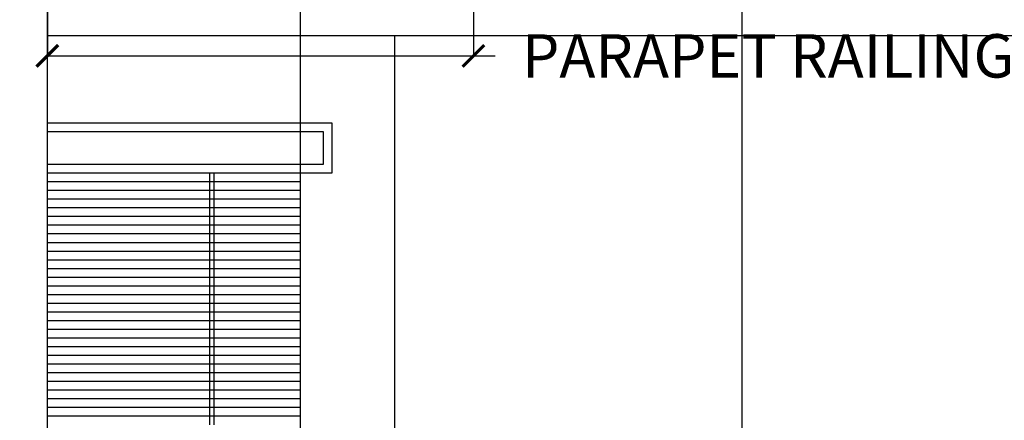
# Model space of a CAD drawing. Units: inches. Extents: x 2278 to 7495, y -71 to 1198.
# Tile 16 of 44: x 4871 to 5007, y 191 to 246. Entities that reach past the tile are written whole.
import ezdxf

# ---------------------------------------------------------------- set-up
doc = ezdxf.new("R2010")
doc.units = ezdxf.units.IN
doc.header["$MEASUREMENT"] = 0
doc.layers.add('A-ANNO-DIMS', color=2, linetype='Continuous', lineweight=18)
doc.layers.add('A-ELEV', color=7, linetype='Continuous', lineweight=25)
doc.styles.get("Standard").update_dxf_attribs({"font": 'arial.ttf'})
doc.dimstyles.get("Standard").update_dxf_attribs({"dimtxt": 6, "dimasz": 3, "dimexe": 0.18, "dimexo": 0.0625, "dimgap": 0.09, "dimtad": 0, "dimtih": 1, "dimtoh": 1, "dimdec": 0, "dimzin": 0, "dimdsep": 46, "dimlunit": 3, "dimtxsty": 'Standard', "dimblk": 'ARCHTICK', "dimcen": 0.09, "dimadec": 0, "dimazin": 0, "dimtfac": 1, "dimtdec": 0, "dimtofl": 0, "dimtmove": 0, "dimatfit": 3, "dimfxl": 1, "dimtolj": 1, "dimtzin": 0, "dimarcsym": 0})

# ---------------------------------------------------------------- blocks, each defined once
blk = doc.blocks.new('_ArchTick')
at = {"color": 0, "linetype": 'ByBlock', "const_width": 0.15}
blk.add_lwpolyline([(-0.5, -0.5), (0.5, 0.5)], dxfattribs=at)
blk = doc.blocks.new('*D57')
at = {"layer": 'A-ANNO-DIMS', "color": 0, "lineweight": -2, "transparency": 16777216}
for p, q in [((4874.68, 250.19), (4874.68, 241.24)), ((4933.56, 250.19), (4933.56, 241.24)), ((4874.68, 241.42), (4933.56, 241.42)), ((4933.56, 241.42), (4936.56, 241.42))]:
    blk.add_line(p, q, dxfattribs=at)
at = {"layer": 'Defpoints', "color": 0, "transparency": 16777216}
for p in [(4874.68, 250.25), (4933.56, 250.25), (4933.56, 241.42)]:
    blk.add_point(p, dxfattribs=at)
at = {"layer": 'A-ANNO-DIMS', "color": 0, "lineweight": -2, "transparency": 16777216, "xscale": 3, "yscale": 3, "zscale": 3, "rotation": 180}
blk.add_blockref('_ArchTick', (4874.68, 241.42), dxfattribs=at)
at = {"layer": 'A-ANNO-DIMS', "color": 0, "lineweight": -2, "transparency": 16777216, "xscale": 3, "yscale": 3, "zscale": 3}
blk.add_blockref('_ArchTick', (4933.56, 241.42), dxfattribs=at)
at = {"layer": 'A-ANNO-DIMS', "color": 0, "transparency": 16777216, "insert": (4995.78, 241.42), "char_height": 6, "attachment_point": 5}
blk.add_mtext('\\A1;PARAPET RAILING 4\'-11" TYP.', dxfattribs=at)
blk = doc.blocks.new('*D123')
at = {"layer": 'A-ANNO-DIMS', "color": 0, "lineweight": -2, "transparency": 16777216}
for p, q in [((4736.95, 340.16), (4736.95, -23.43)), ((5145.68, -1.81), (5145.68, -23.43)), ((4736.95, -23.25), (4923.93, -23.25)), ((5145.68, -23.25), (4958.7, -23.25))]:
    blk.add_line(p, q, dxfattribs=at)
at = {"layer": 'Defpoints', "color": 0, "transparency": 16777216}
for p in [(4736.95, 340.22), (5145.68, -1.75), (5145.68, -23.25)]:
    blk.add_point(p, dxfattribs=at)
at = {"layer": 'A-ANNO-DIMS', "color": 0, "lineweight": -2, "transparency": 16777216, "xscale": 3, "yscale": 3, "zscale": 3, "rotation": 180}
blk.add_blockref('_ArchTick', (4736.95, -23.25), dxfattribs=at)
at = {"layer": 'A-ANNO-DIMS', "color": 0, "lineweight": -2, "transparency": 16777216, "xscale": 3, "yscale": 3, "zscale": 3}
blk.add_blockref('_ArchTick', (5145.68, -23.25), dxfattribs=at)
at = {"layer": 'A-ANNO-DIMS', "color": 0, "transparency": 16777216, "insert": (4941.31, -23.25), "char_height": 6, "attachment_point": 5}
blk.add_mtext('\\A1;34\'-0 1/2"', dxfattribs=at)
blk = doc.blocks.new('*D126')
at = {"layer": 'A-ANNO-DIMS', "color": 0, "lineweight": -2, "transparency": 16777216}
for p, q in [((4837.74, 313.27), (4837.74, 361.9)), ((4837.74, 361.72), (4848.14, 361.72)), ((4874.68, 361.72), (4864.27, 361.72)), ((4874.68, 99.32), (4874.68, 361.9))]:
    blk.add_line(p, q, dxfattribs=at)
at = {"layer": 'Defpoints', "color": 0, "transparency": 16777216}
for p in [(4874.68, 361.72), (4837.74, 313.21), (4874.68, 99.25)]:
    blk.add_point(p, dxfattribs=at)
at = {"layer": 'A-ANNO-DIMS', "color": 0, "lineweight": -2, "transparency": 16777216, "xscale": 3, "yscale": 3, "zscale": 3, "rotation": 180}
blk.add_blockref('_ArchTick', (4837.74, 361.72), dxfattribs=at)
at = {"layer": 'A-ANNO-DIMS', "color": 0, "lineweight": -2, "transparency": 16777216, "xscale": 3, "yscale": 3, "zscale": 3}
blk.add_blockref('_ArchTick', (4874.68, 361.72), dxfattribs=at)
at = {"layer": 'A-ANNO-DIMS', "color": 0, "transparency": 16777216, "insert": (4856.21, 361.72), "char_height": 6, "attachment_point": 5}
blk.add_mtext('\\A1;3\'-1"', dxfattribs=at)
blk = doc.blocks.new('*D127')
at = {"layer": 'A-ANNO-DIMS', "color": 0, "lineweight": -2, "transparency": 16777216}
for p, q in [((4874.68, 99.32), (4874.68, 361.9)), ((4874.68, 361.72), (4881.73, 361.72)), ((4909.68, 361.72), (4902.62, 361.72)), ((4909.68, 99.32), (4909.68, 361.9))]:
    blk.add_line(p, q, dxfattribs=at)
at = {"layer": 'Defpoints', "color": 0, "transparency": 16777216}
for p in [(4909.68, 361.72), (4874.68, 99.25), (4909.68, 99.25)]:
    blk.add_point(p, dxfattribs=at)
at = {"layer": 'A-ANNO-DIMS', "color": 0, "lineweight": -2, "transparency": 16777216, "xscale": 3, "yscale": 3, "zscale": 3, "rotation": 180}
blk.add_blockref('_ArchTick', (4874.68, 361.72), dxfattribs=at)
at = {"layer": 'A-ANNO-DIMS', "color": 0, "lineweight": -2, "transparency": 16777216, "xscale": 3, "yscale": 3, "zscale": 3}
blk.add_blockref('_ArchTick', (4909.68, 361.72), dxfattribs=at)
at = {"layer": 'A-ANNO-DIMS', "color": 0, "transparency": 16777216, "insert": (4892.18, 361.72), "char_height": 6, "attachment_point": 5}
blk.add_mtext('\\A1;2\'-11"', dxfattribs=at)
blk = doc.blocks.new('*D128')
at = {"layer": 'A-ANNO-DIMS', "color": 0, "lineweight": -2, "transparency": 16777216}
for p, q in [((4909.68, 99.32), (4909.68, 361.9)), ((4909.68, 361.72), (4932.11, 361.72)), ((4970.68, 361.72), (4948.24, 361.72)), ((4970.68, 60.78), (4970.68, 361.9))]:
    blk.add_line(p, q, dxfattribs=at)
at = {"layer": 'Defpoints', "color": 0, "transparency": 16777216}
for p in [(4970.68, 361.72), (4909.68, 99.25), (4970.68, 60.72)]:
    blk.add_point(p, dxfattribs=at)
at = {"layer": 'A-ANNO-DIMS', "color": 0, "lineweight": -2, "transparency": 16777216, "xscale": 3, "yscale": 3, "zscale": 3, "rotation": 180}
blk.add_blockref('_ArchTick', (4909.68, 361.72), dxfattribs=at)
at = {"layer": 'A-ANNO-DIMS', "color": 0, "lineweight": -2, "transparency": 16777216, "xscale": 3, "yscale": 3, "zscale": 3}
blk.add_blockref('_ArchTick', (4970.68, 361.72), dxfattribs=at)
at = {"layer": 'A-ANNO-DIMS', "color": 0, "transparency": 16777216, "insert": (4940.18, 361.72), "char_height": 6, "attachment_point": 5}
blk.add_mtext('\\A1;5\'-1"', dxfattribs=at)
blk = doc.blocks.new('*D129')
at = {"layer": 'A-ANNO-DIMS', "color": 0, "lineweight": -2, "transparency": 16777216}
for p, q in [((4970.68, 60.78), (4970.68, 361.9)), ((4970.68, 361.72), (4978.37, 361.72)), ((5016.18, 361.72), (5008.48, 361.72)), ((5016.18, 99.32), (5016.18, 361.9))]:
    blk.add_line(p, q, dxfattribs=at)
at = {"layer": 'Defpoints', "color": 0, "transparency": 16777216}
for p in [(5016.18, 361.72), (5016.18, 99.25), (4970.68, 60.72)]:
    blk.add_point(p, dxfattribs=at)
at = {"layer": 'A-ANNO-DIMS', "color": 0, "lineweight": -2, "transparency": 16777216, "xscale": 3, "yscale": 3, "zscale": 3, "rotation": 180}
blk.add_blockref('_ArchTick', (4970.68, 361.72), dxfattribs=at)
at = {"layer": 'A-ANNO-DIMS', "color": 0, "lineweight": -2, "transparency": 16777216, "xscale": 3, "yscale": 3, "zscale": 3}
blk.add_blockref('_ArchTick', (5016.18, 361.72), dxfattribs=at)
at = {"layer": 'A-ANNO-DIMS', "color": 0, "transparency": 16777216, "insert": (4993.43, 361.72), "char_height": 6, "attachment_point": 5}
blk.add_mtext('\\A1;3\'-9 1/2"', dxfattribs=at)

msp = doc.modelspace()

# ---------------------------------------------------------------- linework, layer by layer
at = {"layer": 'A-ELEV'}
for p, q in [((4874.68, 124.25), (4874.68, 250.25)), ((4874.68, 244.25), (5145.68, 244.25)), ((4922.68, 66.66), (4922.68, 244.25)), ((4970.68, 160.25), (4970.68, 244.25)), ((4874.68, 225.25), (4909.68, 225.25)), ((4897.08, 225.25), (4897.08, 190.45)), ((4897.08, 225.25), (4897.08, 191.65)), ((4897.08, 225.25), (4897.08, 191.65)), ((4897.08, 225.25), (4897.08, 191.65)), ((4897.68, 225.25), (4897.68, 190.45)), ((4897.68, 225.25), (4897.68, 191.65)), ((4897.68, 225.25), (4897.68, 191.65)), ((4897.68, 225.25), (4897.68, 191.65)), ((4909.68, 190.45), (4909.68, 225.25)), ((4874.68, 224.05), (4909.68, 224.05)), ((4874.68, 222.85), (4909.68, 222.85)), ((4874.68, 221.65), (4909.68, 221.65)), ((4874.68, 220.45), (4909.68, 220.45)), ((4874.68, 219.25), (4909.68, 219.25)), ((4874.68, 218.05), (4909.68, 218.05)), ((4874.68, 216.85), (4909.68, 216.85)), ((4874.68, 215.65), (4909.68, 215.65)), ((4874.68, 214.45), (4909.68, 214.45)), ((4874.68, 213.25), (4909.68, 213.25)), ((4874.68, 212.05), (4909.68, 212.05)), ((4874.68, 210.85), (4909.68, 210.85)), ((4874.68, 209.65), (4909.68, 209.65)), ((4874.68, 208.45), (4909.68, 208.45)), ((4874.68, 207.25), (4909.68, 207.25)), ((4874.68, 206.05), (4909.68, 206.05)), ((4874.68, 204.85), (4909.68, 204.85)), ((4874.68, 203.65), (4909.68, 203.65)), ((4874.68, 202.45), (4909.68, 202.45)), ((4874.68, 201.25), (4909.68, 201.25)), ((4874.68, 200.05), (4909.68, 200.05)), ((4874.68, 198.85), (4909.68, 198.85)), ((4874.68, 197.65), (4909.68, 197.65)), ((4874.68, 196.45), (4909.68, 196.45)), ((4874.68, 195.25), (4909.68, 195.25)), ((4874.68, 194.05), (4909.68, 194.05)), ((4874.68, 192.85), (4909.68, 192.85)), ((4874.68, 191.65), (4909.68, 191.65))]:
    msp.add_line(p, q, dxfattribs=at)
for points in [[(4874.68, 225.25), (4914.03, 225.25), (4914.03, 232.1), (4874.68, 232.1)], [(4874.68, 226.45), (4912.83, 226.45), (4912.83, 230.9), (4874.68, 230.9)]]:
    msp.add_lwpolyline(points, dxfattribs=at)

# ---------------------------------------------------------------- dimensions: what is measured, and where the dimension line sits
at = {"layer": 'A-ANNO-DIMS'}
for base, p1, p2, picture, middle in [((5016.18, 361.72), (4970.68, 60.72), (5016.18, 99.25), '*D129', (4993.43, 361.72)), ((4874.68, 361.72), (4837.74, 313.21), (4874.68, 99.25), '*D126', (4856.21, 361.72)), ((4909.68, 361.72), (4874.68, 99.25), (4909.68, 99.25), '*D127', (4892.18, 361.72)), ((4970.68, 361.72), (4909.68, 99.25), (4970.68, 60.72), '*D128', (4940.18, 361.72)), ((5145.68, -23.25), (4736.95, 340.22), (5145.68, -1.75), '*D123', (4941.31, -23.25))]:
    dim = msp.add_linear_dim(base=base, p1=p1, p2=p2, dimstyle='Standard', override={"dimdec": 1, "dimlfac": 1, "dimrnd": 0, "dimzin": 1, "dimdsep": 46, "dimlunit": 4, "dimfrac": 2}, dxfattribs=at)
    dim.commit()
    dim.dimension.update_dxf_attribs({"geometry": picture, "text_midpoint": middle})
dim = msp.add_linear_dim(base=(4933.56, 241.42), p1=(4874.68, 250.25), p2=(4933.56, 250.25), text='PARAPET RAILING <> TYP.', dimstyle='Standard', override={"dimdec": 1, "dimrnd": 0, "dimzin": 1, "dimlunit": 4, "dimfrac": 2}, dxfattribs=at)
dim.commit()
dim.dimension.update_dxf_attribs({"geometry": '*D57', "text_midpoint": (4995.78, 241.42)})

doc.saveas('drawing.dxf')
